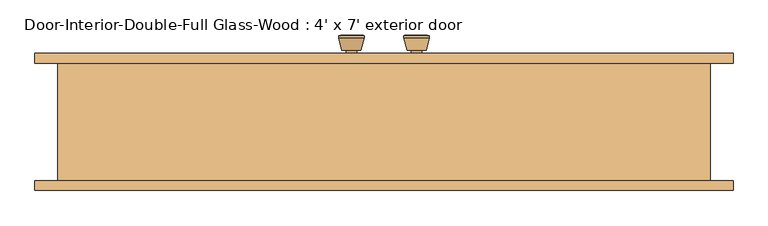
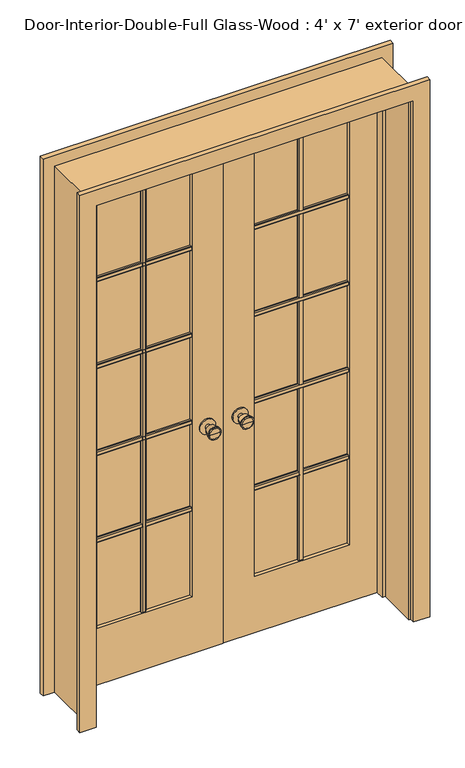
"""IFC4 building model written with IfcOpenShell, lengths in millimetres: door geometry, Door-Interior-Double-Full Glass-Wood : 4' x 7' exterior door."""

from ifc_helpers import new_model, si_unit, point, frame, frame_2d, origin, place, context, project, spatial, polyline, circle_curve, trimmed, segment, composite_curve, outline, extrude, faceted_brep, source, transform, mapped, element, save
from ifc_brep_helpers import plane_surface, cylinder_surface, revolved_surface, advanced_brep


def door_interior_double_full_glass_wood_4_x_7_exterior_door_6b6f14de(model_context):
    return source(origin(), model_context, "Body", "SolidModel", [
        advanced_brep(
        [(-63.5, 117.125, 914.4), (-73.5, 117.125, 914.4), (-53.5, 117.125, 914.4), (-83.9758676, 166.125, 914.4), (-63.5, 166.125, 914.4), (-43.0241324, 166.125, 914.4), (-88.5, 164.2971319, 914.4), (-38.5, 164.2971319, 914.4), (-88.5, 160.8334537, 914.4), (-38.5, 160.8334537, 914.4), (-82.136236, 136.125, 914.4), (-44.863764, 136.125, 914.4), (-73.5, 136.125, 914.4), (-53.5, 136.125, 914.4)],
        [
            (0, 1),
            (1, 2, circle_curve(frame((-63.5, 117.125, 914.4), z_axis=(0.0, -1.0, 0.0), x_axis=(1.0, 0.0, 0.0)), 10.0)),
            (2, 0),
            (2, 1, circle_curve(frame((-63.5, 117.125, 914.4), z_axis=(0.0, -1.0, 0.0), x_axis=(1.0, 0.0, 0.0)), 10.0)),
            (3, 4),
            (4, 5),
            (5, 3, circle_curve(frame((-63.5, 166.125, 914.4), z_axis=(0.0, 1.0, 0.0), x_axis=(1.0, 0.0, 0.0)), 20.4758676)),
            (3, 5, circle_curve(frame((-63.5, 166.125, 914.4), z_axis=(0.0, 1.0, 0.0), x_axis=(1.0, 0.0, 0.0)), 20.4758676)),
            (6, 3),
            (5, 7),
            (7, 6, circle_curve(frame((-63.5, 164.2971319, 914.4), z_axis=(0.0, 1.0, 0.0), x_axis=(1.0, 0.0, 0.0)), 25.0)),
            (6, 7, circle_curve(frame((-63.5, 164.2971319, 914.4), z_axis=(0.0, 1.0, 0.0), x_axis=(1.0, 0.0, 0.0)), 25.0)),
            (8, 6),
            (7, 9),
            (9, 8, circle_curve(frame((-63.5, 160.8334537, 914.4), z_axis=(0.0, 1.0, 0.0), x_axis=(1.0, 0.0, 0.0)), 25.0)),
            (8, 9, circle_curve(frame((-63.5, 160.8334537, 914.4), z_axis=(0.0, 1.0, 0.0), x_axis=(1.0, 0.0, 0.0)), 25.0)),
            (10, 8),
            (9, 11),
            (11, 10, circle_curve(frame((-63.5, 136.125, 914.4), z_axis=(0.0, 1.0, 0.0), x_axis=(1.0, 0.0, 0.0)), 18.636236)),
            (10, 11, circle_curve(frame((-63.5, 136.125, 914.4), z_axis=(0.0, 1.0, 0.0), x_axis=(1.0, 0.0, 0.0)), 18.636236)),
            (12, 10),
            (11, 13),
            (13, 12, circle_curve(frame((-63.5, 136.125, 914.4), z_axis=(0.0, 1.0, 0.0), x_axis=(1.0, 0.0, 0.0)), 10.0)),
            (12, 13, circle_curve(frame((-63.5, 136.125, 914.4), z_axis=(0.0, 1.0, 0.0), x_axis=(1.0, 0.0, 0.0)), 10.0)),
            (1, 12),
            (13, 2),
        ],
        [
            plane_surface(frame((-63.5, 117.125, 914.4), z_axis=(0.0, -1.0, 0.0), x_axis=(1.0, 0.0, 0.0))),
            plane_surface(frame((-63.5, 166.125, 914.4), z_axis=(0.0, 1.0, 0.0), x_axis=(1.0, 0.0, 0.0))),
            revolved_surface(polyline([(-43.0241324, 166.125, 914.4), (-38.5, 164.2971319, 914.4)]), (-63.5, 117.125, 914.4), (0.0, -1.0, 0.0)),
            cylinder_surface(frame((-63.5, 117.125, 914.4), z_axis=(0.0, -1.0, 0.0), x_axis=(1.0, 0.0, 0.0)), 25.0),
            revolved_surface(polyline([(-38.5, 160.8334537, 914.4), (-44.863764, 136.125, 914.4)]), (-63.5, 117.125, 914.4), (0.0, -1.0, 0.0)),
            plane_surface(frame((-63.5, 136.125, 914.4), z_axis=(0.0, -1.0, 0.0), x_axis=(1.0, 0.0, 0.0))),
            cylinder_surface(frame((-63.5, 117.125, 914.4), z_axis=(0.0, -1.0, 0.0), x_axis=(1.0, 0.0, 0.0)), 10.0),
        ],
        [
            (0, [[1, 2, 3]]),
            (0, [[-3, 4, -1]]),
            (1, [[5, 6, 7]]),
            (1, [[-6, -5, 8]]),
            (2, [[9, -7, 10, 11]]),
            (2, [[-10, -8, -9, 12]]),
            (3, [[13, -11, 14, 15]]),
            (3, [[-14, -12, -13, 16]]),
            (4, [[17, -15, 18, 19]]),
            (4, [[-18, -16, -17, 20]]),
            (5, [[21, -19, 22, 23]]),
            (5, [[-22, -20, -21, 24]]),
            (6, [[25, -23, 26, -2]]),
            (6, [[-26, -24, -25, -4]]),
        ],
    ),
        extrude(outline(composite_curve([segment(trimmed(circle_curve(frame_2d((914.4, -63.5)), 30.0), [point((914.4, -33.5))], [point((914.4, -93.5))], False, "CARTESIAN"), True, "CONTINUOUS"), segment(trimmed(circle_curve(frame_2d((914.4, -63.5)), 30.0), [point((914.4, -93.5))], [point((914.4, -33.5))], False, "CARTESIAN"), True, "CONTINUOUS")], self_intersect=False)), frame((0.0, 111.125, 0.0), z_axis=(0.0, 1.0, 0.0), x_axis=(0.0, 0.0, 1.0)), (0.0, 0.0, 1.0), 6.0),
        advanced_brep(
        [(-63.5, 70.2, 914.4), (-53.5, 70.2, 914.4), (-73.5, 70.2, 914.4), (-83.9758676, 21.2, 914.4), (-43.0241324, 21.2, 914.4), (-63.5, 21.2, 914.4), (-88.5, 23.0278681, 914.4), (-38.5, 23.0278681, 914.4), (-88.5, 26.4915463, 914.4), (-38.5, 26.4915463, 914.4), (-82.136236, 51.2, 914.4), (-44.863764, 51.2, 914.4), (-73.5, 51.2, 914.4), (-53.5, 51.2, 914.4)],
        [
            (0, 1),
            (1, 2, circle_curve(frame((-63.5, 70.2, 914.4), z_axis=(0.0, 1.0, 0.0), x_axis=(1.0, 0.0, 0.0)), 10.0)),
            (2, 0),
            (2, 1, circle_curve(frame((-63.5, 70.2, 914.4), z_axis=(0.0, 1.0, 0.0), x_axis=(1.0, 0.0, 0.0)), 10.0)),
            (3, 4, circle_curve(frame((-63.5, 21.2, 914.4), z_axis=(0.0, -1.0, 0.0), x_axis=(1.0, 0.0, 0.0)), 20.4758676)),
            (4, 5),
            (5, 3),
            (4, 3, circle_curve(frame((-63.5, 21.2, 914.4), z_axis=(0.0, -1.0, 0.0), x_axis=(1.0, 0.0, 0.0)), 20.4758676)),
            (6, 7, circle_curve(frame((-63.5, 23.0278681, 914.4), z_axis=(0.0, -1.0, 0.0), x_axis=(1.0, 0.0, 0.0)), 25.0)),
            (7, 4),
            (3, 6),
            (7, 6, circle_curve(frame((-63.5, 23.0278681, 914.4), z_axis=(0.0, -1.0, 0.0), x_axis=(1.0, 0.0, 0.0)), 25.0)),
            (8, 9, circle_curve(frame((-63.5, 26.4915463, 914.4), z_axis=(0.0, -1.0, 0.0), x_axis=(1.0, 0.0, 0.0)), 25.0)),
            (9, 7),
            (6, 8),
            (9, 8, circle_curve(frame((-63.5, 26.4915463, 914.4), z_axis=(0.0, -1.0, 0.0), x_axis=(1.0, 0.0, 0.0)), 25.0)),
            (10, 11, circle_curve(frame((-63.5, 51.2, 914.4), z_axis=(0.0, -1.0, 0.0), x_axis=(1.0, 0.0, 0.0)), 18.636236)),
            (11, 9),
            (8, 10),
            (11, 10, circle_curve(frame((-63.5, 51.2, 914.4), z_axis=(0.0, -1.0, 0.0), x_axis=(1.0, 0.0, 0.0)), 18.636236)),
            (12, 13, circle_curve(frame((-63.5, 51.2, 914.4), z_axis=(0.0, -1.0, 0.0), x_axis=(1.0, 0.0, 0.0)), 10.0)),
            (13, 11),
            (10, 12),
            (13, 12, circle_curve(frame((-63.5, 51.2, 914.4), z_axis=(0.0, -1.0, 0.0), x_axis=(1.0, 0.0, 0.0)), 10.0)),
            (1, 13),
            (12, 2),
        ],
        [
            plane_surface(frame((-63.5, 70.2, 914.4), z_axis=(0.0, 1.0, 0.0), x_axis=(1.0, 0.0, 0.0))),
            plane_surface(frame((-63.5, 21.2, 914.4), z_axis=(0.0, -1.0, 0.0), x_axis=(1.0, 0.0, 0.0))),
            revolved_surface(polyline([(-43.0241324, 21.2, 914.4), (-38.5, 23.0278681, 914.4)]), (-63.5, 70.2, 914.4), (0.0, 1.0, 0.0)),
            cylinder_surface(frame((-63.5, 70.2, 914.4), z_axis=(0.0, 1.0, 0.0), x_axis=(1.0, 0.0, 0.0)), 25.0),
            revolved_surface(polyline([(-38.5, 26.4915463, 914.4), (-44.863764, 51.2, 914.4)]), (-63.5, 70.2, 914.4), (0.0, 1.0, 0.0)),
            plane_surface(frame((-63.5, 51.2, 914.4), z_axis=(0.0, 1.0, 0.0), x_axis=(1.0, 0.0, 0.0))),
            cylinder_surface(frame((-63.5, 70.2, 914.4), z_axis=(0.0, 1.0, 0.0), x_axis=(1.0, 0.0, 0.0)), 10.0),
        ],
        [
            (0, [[1, 2, 3]]),
            (0, [[-3, 4, -1]]),
            (1, [[5, 6, 7]]),
            (1, [[8, -7, -6]]),
            (2, [[9, 10, -5, 11]]),
            (2, [[12, -11, -8, -10]]),
            (3, [[13, 14, -9, 15]]),
            (3, [[16, -15, -12, -14]]),
            (4, [[17, 18, -13, 19]]),
            (4, [[20, -19, -16, -18]]),
            (5, [[21, 22, -17, 23]]),
            (5, [[24, -23, -20, -22]]),
            (6, [[-2, 25, -21, 26]]),
            (6, [[-4, -26, -24, -25]]),
        ],
    ),
        extrude(outline(composite_curve([segment(trimmed(circle_curve(frame_2d((914.4, -63.5)), 30.0), [point((914.4, -33.5))], [point((914.4, -93.5))], False, "CARTESIAN"), True, "CONTINUOUS"), segment(trimmed(circle_curve(frame_2d((914.4, -63.5)), 30.0), [point((914.4, -93.5))], [point((914.4, -33.5))], False, "CARTESIAN"), True, "CONTINUOUS")], self_intersect=False)), frame((0.0, 70.2, 0.0), z_axis=(0.0, 1.0, 0.0), x_axis=(0.0, 0.0, 1.0)), (0.0, 0.0, 1.0), 6.0),
        extrude(outline(polyline([(90.17, 1667.51), (90.17, 1648.46), (83.82, 1648.46), (80.645, 1651.635), (80.645, 1664.335), (83.82, 1667.51), (90.17, 1667.51)])), frame((120.65, 0.0, 0.0), z_axis=(1.0, 0.0, 0.0), x_axis=(0.0, 1.0, 0.0)), (0.0, 0.0, 1.0), 368.3),
        extrude(outline(polyline([(90.17, 1310.9575), (90.17, 1291.9075), (83.82, 1291.9075), (80.645, 1295.0825), (80.645, 1307.7825), (83.82, 1310.9575), (90.17, 1310.9575)])), frame((120.65, 0.0, 0.0), z_axis=(1.0, 0.0, 0.0), x_axis=(0.0, 1.0, 0.0)), (0.0, 0.0, 1.0), 368.3),
        extrude(outline(polyline([(90.17, 954.405), (90.17, 935.355), (83.82, 935.355), (80.645, 938.53), (80.645, 951.23), (83.82, 954.405), (90.17, 954.405)])), frame((120.65, 0.0, 0.0), z_axis=(1.0, 0.0, 0.0), x_axis=(0.0, 1.0, 0.0)), (0.0, 0.0, 1.0), 368.3),
        extrude(outline(polyline([(295.275, 90.17), (314.325, 90.17), (314.325, 83.82), (311.15, 80.645), (298.45, 80.645), (295.275, 83.82), (295.275, 90.17)])), frame((0.0, 0.0, 231.775), z_axis=(0.0, 0.0, 1.0), x_axis=(1.0, 0.0, 0.0)), (0.0, 0.0, 1.0), 1782.7625),
        extrude(outline(polyline([(90.17, 597.8525), (90.17, 578.8025), (83.82, 578.8025), (80.645, 581.9775), (80.645, 594.6775), (83.82, 597.8525), (90.17, 597.8525)])), frame((120.65, 0.0, 0.0), z_axis=(1.0, 0.0, 0.0), x_axis=(0.0, 1.0, 0.0)), (0.0, 0.0, 1.0), 368.3),
        extrude(outline(polyline([(97.155, 1667.51), (103.505, 1667.51), (106.68, 1664.335), (106.68, 1651.635), (103.505, 1648.46), (97.155, 1648.46), (97.155, 1667.51)])), frame((-488.95, 0.0, 0.0), z_axis=(1.0, 0.0, 0.0), x_axis=(0.0, 1.0, 0.0)), (0.0, 0.0, 1.0), 368.3),
        extrude(outline(polyline([(97.155, 1310.9575), (103.505, 1310.9575), (106.68, 1307.7825), (106.68, 1295.0825), (103.505, 1291.9075), (97.155, 1291.9075), (97.155, 1310.9575)])), frame((-488.95, 0.0, 0.0), z_axis=(1.0, 0.0, 0.0), x_axis=(0.0, 1.0, 0.0)), (0.0, 0.0, 1.0), 368.3),
        extrude(outline(polyline([(97.155, 954.405), (103.505, 954.405), (106.68, 951.23), (106.68, 938.53), (103.505, 935.355), (97.155, 935.355), (97.155, 954.405)])), frame((-488.95, 0.0, 0.0), z_axis=(1.0, 0.0, 0.0), x_axis=(0.0, 1.0, 0.0)), (0.0, 0.0, 1.0), 368.3),
        extrude(outline(polyline([(-314.325, 97.155), (-314.325, 103.505), (-311.15, 106.68), (-298.45, 106.68), (-295.275, 103.505), (-295.275, 97.155), (-314.325, 97.155)])), frame((0.0, 0.0, 231.775), z_axis=(0.0, 0.0, 1.0), x_axis=(1.0, 0.0, 0.0)), (0.0, 0.0, 1.0), 1782.7625),
        extrude(outline(polyline([(97.155, 597.8525), (103.505, 597.8525), (106.68, 594.6775), (106.68, 581.9775), (103.505, 578.8025), (97.155, 578.8025), (97.155, 597.8525)])), frame((-488.95, 0.0, 0.0), z_axis=(1.0, 0.0, 0.0), x_axis=(0.0, 1.0, 0.0)), (0.0, 0.0, 1.0), 368.3),
        extrude(outline(polyline([(97.155, 1667.51), (103.505, 1667.51), (106.68, 1664.335), (106.68, 1651.635), (103.505, 1648.46), (97.155, 1648.46), (97.155, 1667.51)])), frame((120.65, 0.0, 0.0), z_axis=(1.0, 0.0, 0.0), x_axis=(0.0, 1.0, 0.0)), (0.0, 0.0, 1.0), 368.3),
        extrude(outline(polyline([(97.155, 1310.9575), (103.505, 1310.9575), (106.68, 1307.7825), (106.68, 1295.0825), (103.505, 1291.9075), (97.155, 1291.9075), (97.155, 1310.9575)])), frame((120.65, 0.0, 0.0), z_axis=(1.0, 0.0, 0.0), x_axis=(0.0, 1.0, 0.0)), (0.0, 0.0, 1.0), 368.3),
        extrude(outline(polyline([(97.155, 954.405), (103.505, 954.405), (106.68, 951.23), (106.68, 938.53), (103.505, 935.355), (97.155, 935.355), (97.155, 954.405)])), frame((120.65, 0.0, 0.0), z_axis=(1.0, 0.0, 0.0), x_axis=(0.0, 1.0, 0.0)), (0.0, 0.0, 1.0), 368.3),
        extrude(outline(polyline([(295.275, 97.155), (295.275, 103.505), (298.45, 106.68), (311.15, 106.68), (314.325, 103.505), (314.325, 97.155), (295.275, 97.155)])), frame((0.0, 0.0, 231.775), z_axis=(0.0, 0.0, 1.0), x_axis=(1.0, 0.0, 0.0)), (0.0, 0.0, 1.0), 1782.7625),
        extrude(outline(polyline([(97.155, 597.8525), (103.505, 597.8525), (106.68, 594.6775), (106.68, 581.9775), (103.505, 578.8025), (97.155, 578.8025), (97.155, 597.8525)])), frame((120.65, 0.0, 0.0), z_axis=(1.0, 0.0, 0.0), x_axis=(0.0, 1.0, 0.0)), (0.0, 0.0, 1.0), 368.3),
        extrude(outline(polyline([(90.17, 1667.51), (90.17, 1648.46), (83.82, 1648.46), (80.645, 1651.635), (80.645, 1664.335), (83.82, 1667.51), (90.17, 1667.51)])), frame((-488.95, 0.0, 0.0), z_axis=(1.0, 0.0, 0.0), x_axis=(0.0, 1.0, 0.0)), (0.0, 0.0, 1.0), 368.3),
        extrude(outline(polyline([(90.17, 1310.9575), (90.17, 1291.9075), (83.82, 1291.9075), (80.645, 1295.0825), (80.645, 1307.7825), (83.82, 1310.9575), (90.17, 1310.9575)])), frame((-488.95, 0.0, 0.0), z_axis=(1.0, 0.0, 0.0), x_axis=(0.0, 1.0, 0.0)), (0.0, 0.0, 1.0), 368.3),
        extrude(outline(polyline([(90.17, 954.405), (90.17, 935.355), (83.82, 935.355), (80.645, 938.53), (80.645, 951.23), (83.82, 954.405), (90.17, 954.405)])), frame((-488.95, 0.0, 0.0), z_axis=(1.0, 0.0, 0.0), x_axis=(0.0, 1.0, 0.0)), (0.0, 0.0, 1.0), 368.3),
        extrude(outline(polyline([(-314.325, 90.17), (-295.275, 90.17), (-295.275, 83.82), (-298.45, 80.645), (-311.15, 80.645), (-314.325, 83.82), (-314.325, 90.17)])), frame((0.0, 0.0, 231.775), z_axis=(0.0, 0.0, 1.0), x_axis=(1.0, 0.0, 0.0)), (0.0, 0.0, 1.0), 1782.7625),
        extrude(outline(polyline([(90.17, 597.8525), (90.17, 578.8025), (83.82, 578.8025), (80.645, 581.9775), (80.645, 594.6775), (83.82, 597.8525), (90.17, 597.8525)])), frame((-488.95, 0.0, 0.0), z_axis=(1.0, 0.0, 0.0), x_axis=(0.0, 1.0, 0.0)), (0.0, 0.0, 1.0), 368.3),
        advanced_brep(
        [(63.5, 70.2, 914.4), (73.5, 70.2, 914.4), (53.5, 70.2, 914.4), (83.9758676, 21.2, 914.4), (63.5, 21.2, 914.4), (43.0241324, 21.2, 914.4), (88.5, 23.0278681, 914.4), (38.5, 23.0278681, 914.4), (88.5, 26.4915463, 914.4), (38.5, 26.4915463, 914.4), (82.136236, 51.2, 914.4), (44.863764, 51.2, 914.4), (73.5, 51.2, 914.4), (53.5, 51.2, 914.4)],
        [
            (0, 1),
            (1, 2, circle_curve(frame((63.5, 70.2, 914.4), z_axis=(0.0, 1.0, 0.0), x_axis=(-1.0, 0.0, 0.0)), 10.0)),
            (2, 0),
            (2, 1, circle_curve(frame((63.5, 70.2, 914.4), z_axis=(0.0, 1.0, 0.0), x_axis=(-1.0, 0.0, 0.0)), 10.0)),
            (3, 4),
            (4, 5),
            (5, 3, circle_curve(frame((63.5, 21.2, 914.4), z_axis=(0.0, -1.0, 0.0), x_axis=(-1.0, 0.0, 0.0)), 20.4758676)),
            (3, 5, circle_curve(frame((63.5, 21.2, 914.4), z_axis=(0.0, -1.0, 0.0), x_axis=(-1.0, 0.0, 0.0)), 20.4758676)),
            (6, 3),
            (5, 7),
            (7, 6, circle_curve(frame((63.5, 23.0278681, 914.4), z_axis=(0.0, -1.0, 0.0), x_axis=(-1.0, 0.0, 0.0)), 25.0)),
            (6, 7, circle_curve(frame((63.5, 23.0278681, 914.4), z_axis=(0.0, -1.0, 0.0), x_axis=(-1.0, 0.0, 0.0)), 25.0)),
            (8, 6),
            (7, 9),
            (9, 8, circle_curve(frame((63.5, 26.4915463, 914.4), z_axis=(0.0, -1.0, 0.0), x_axis=(-1.0, 0.0, 0.0)), 25.0)),
            (8, 9, circle_curve(frame((63.5, 26.4915463, 914.4), z_axis=(0.0, -1.0, 0.0), x_axis=(-1.0, 0.0, 0.0)), 25.0)),
            (10, 8),
            (9, 11),
            (11, 10, circle_curve(frame((63.5, 51.2, 914.4), z_axis=(0.0, -1.0, 0.0), x_axis=(-1.0, 0.0, 0.0)), 18.636236)),
            (10, 11, circle_curve(frame((63.5, 51.2, 914.4), z_axis=(0.0, -1.0, 0.0), x_axis=(-1.0, 0.0, 0.0)), 18.636236)),
            (12, 10),
            (11, 13),
            (13, 12, circle_curve(frame((63.5, 51.2, 914.4), z_axis=(0.0, -1.0, 0.0), x_axis=(-1.0, 0.0, 0.0)), 10.0)),
            (12, 13, circle_curve(frame((63.5, 51.2, 914.4), z_axis=(0.0, -1.0, 0.0), x_axis=(-1.0, 0.0, 0.0)), 10.0)),
            (1, 12),
            (13, 2),
        ],
        [
            plane_surface(frame((63.5, 70.2, 914.4), z_axis=(0.0, 1.0, 0.0), x_axis=(-1.0, 0.0, 0.0))),
            plane_surface(frame((63.5, 21.2, 914.4), z_axis=(0.0, -1.0, 0.0), x_axis=(-1.0, 0.0, 0.0))),
            revolved_surface(polyline([(43.0241324, 21.2, 914.4), (38.5, 23.0278681, 914.4)]), (63.5, 70.2, 914.4), (0.0, 1.0, 0.0)),
            cylinder_surface(frame((63.5, 70.2, 914.4), z_axis=(0.0, 1.0, 0.0), x_axis=(-1.0, 0.0, 0.0)), 25.0),
            revolved_surface(polyline([(38.5, 26.4915463, 914.4), (44.863764, 51.2, 914.4)]), (63.5, 70.2, 914.4), (0.0, 1.0, 0.0)),
            plane_surface(frame((63.5, 51.2, 914.4), z_axis=(0.0, 1.0, 0.0), x_axis=(-1.0, 0.0, 0.0))),
            cylinder_surface(frame((63.5, 70.2, 914.4), z_axis=(0.0, 1.0, 0.0), x_axis=(-1.0, 0.0, 0.0)), 10.0),
        ],
        [
            (0, [[1, 2, 3]]),
            (0, [[-3, 4, -1]]),
            (1, [[5, 6, 7]]),
            (1, [[-6, -5, 8]]),
            (2, [[9, -7, 10, 11]]),
            (2, [[-10, -8, -9, 12]]),
            (3, [[13, -11, 14, 15]]),
            (3, [[-14, -12, -13, 16]]),
            (4, [[17, -15, 18, 19]]),
            (4, [[-18, -16, -17, 20]]),
            (5, [[21, -19, 22, 23]]),
            (5, [[-22, -20, -21, 24]]),
            (6, [[25, -23, 26, -2]]),
            (6, [[-26, -24, -25, -4]]),
        ],
    ),
        extrude(outline(composite_curve([segment(trimmed(circle_curve(frame_2d((914.4, 63.5)), 30.0), [point((914.4, 33.5))], [point((914.4, 93.5))], False, "CARTESIAN"), True, "CONTINUOUS"), segment(trimmed(circle_curve(frame_2d((914.4, 63.5)), 30.0), [point((914.4, 93.5))], [point((914.4, 33.5))], False, "CARTESIAN"), True, "CONTINUOUS")], self_intersect=False)), frame((0.0, 70.2, 0.0), z_axis=(0.0, 1.0, 0.0), x_axis=(0.0, 0.0, 1.0)), (0.0, 0.0, 1.0), 6.0),
        advanced_brep(
        [(63.5, 117.125, 914.4), (53.5, 117.125, 914.4), (73.5, 117.125, 914.4), (83.9758676, 166.125, 914.4), (43.0241324, 166.125, 914.4), (63.5, 166.125, 914.4), (88.5, 164.2971319, 914.4), (38.5, 164.2971319, 914.4), (88.5, 160.8334537, 914.4), (38.5, 160.8334537, 914.4), (82.136236, 136.125, 914.4), (44.863764, 136.125, 914.4), (73.5, 136.125, 914.4), (53.5, 136.125, 914.4)],
        [
            (0, 1),
            (1, 2, circle_curve(frame((63.5, 117.125, 914.4), z_axis=(0.0, -1.0, 0.0), x_axis=(-1.0, 0.0, 0.0)), 10.0)),
            (2, 0),
            (2, 1, circle_curve(frame((63.5, 117.125, 914.4), z_axis=(0.0, -1.0, 0.0), x_axis=(-1.0, 0.0, 0.0)), 10.0)),
            (3, 4, circle_curve(frame((63.5, 166.125, 914.4), z_axis=(0.0, 1.0, 0.0), x_axis=(-1.0, 0.0, 0.0)), 20.4758676)),
            (4, 5),
            (5, 3),
            (4, 3, circle_curve(frame((63.5, 166.125, 914.4), z_axis=(0.0, 1.0, 0.0), x_axis=(-1.0, 0.0, 0.0)), 20.4758676)),
            (6, 7, circle_curve(frame((63.5, 164.2971319, 914.4), z_axis=(0.0, 1.0, 0.0), x_axis=(-1.0, 0.0, 0.0)), 25.0)),
            (7, 4),
            (3, 6),
            (7, 6, circle_curve(frame((63.5, 164.2971319, 914.4), z_axis=(0.0, 1.0, 0.0), x_axis=(-1.0, 0.0, 0.0)), 25.0)),
            (8, 9, circle_curve(frame((63.5, 160.8334537, 914.4), z_axis=(0.0, 1.0, 0.0), x_axis=(-1.0, 0.0, 0.0)), 25.0)),
            (9, 7),
            (6, 8),
            (9, 8, circle_curve(frame((63.5, 160.8334537, 914.4), z_axis=(0.0, 1.0, 0.0), x_axis=(-1.0, 0.0, 0.0)), 25.0)),
            (10, 11, circle_curve(frame((63.5, 136.125, 914.4), z_axis=(0.0, 1.0, 0.0), x_axis=(-1.0, 0.0, 0.0)), 18.636236)),
            (11, 9),
            (8, 10),
            (11, 10, circle_curve(frame((63.5, 136.125, 914.4), z_axis=(0.0, 1.0, 0.0), x_axis=(-1.0, 0.0, 0.0)), 18.636236)),
            (12, 13, circle_curve(frame((63.5, 136.125, 914.4), z_axis=(0.0, 1.0, 0.0), x_axis=(-1.0, 0.0, 0.0)), 10.0)),
            (13, 11),
            (10, 12),
            (13, 12, circle_curve(frame((63.5, 136.125, 914.4), z_axis=(0.0, 1.0, 0.0), x_axis=(-1.0, 0.0, 0.0)), 10.0)),
            (1, 13),
            (12, 2),
        ],
        [
            plane_surface(frame((63.5, 117.125, 914.4), z_axis=(0.0, -1.0, 0.0), x_axis=(-1.0, 0.0, 0.0))),
            plane_surface(frame((63.5, 166.125, 914.4), z_axis=(0.0, 1.0, 0.0), x_axis=(-1.0, 0.0, 0.0))),
            revolved_surface(polyline([(43.0241324, 166.125, 914.4), (38.5, 164.2971319, 914.4)]), (63.5, 117.125, 914.4), (0.0, -1.0, 0.0)),
            cylinder_surface(frame((63.5, 117.125, 914.4), z_axis=(0.0, -1.0, 0.0), x_axis=(-1.0, 0.0, 0.0)), 25.0),
            revolved_surface(polyline([(38.5, 160.8334537, 914.4), (44.863764, 136.125, 914.4)]), (63.5, 117.125, 914.4), (0.0, -1.0, 0.0)),
            plane_surface(frame((63.5, 136.125, 914.4), z_axis=(0.0, -1.0, 0.0), x_axis=(-1.0, 0.0, 0.0))),
            cylinder_surface(frame((63.5, 117.125, 914.4), z_axis=(0.0, -1.0, 0.0), x_axis=(-1.0, 0.0, 0.0)), 10.0),
        ],
        [
            (0, [[1, 2, 3]]),
            (0, [[-3, 4, -1]]),
            (1, [[5, 6, 7]]),
            (1, [[8, -7, -6]]),
            (2, [[9, 10, -5, 11]]),
            (2, [[12, -11, -8, -10]]),
            (3, [[13, 14, -9, 15]]),
            (3, [[16, -15, -12, -14]]),
            (4, [[17, 18, -13, 19]]),
            (4, [[20, -19, -16, -18]]),
            (5, [[21, 22, -17, 23]]),
            (5, [[24, -23, -20, -22]]),
            (6, [[-2, 25, -21, 26]]),
            (6, [[-4, -26, -24, -25]]),
        ],
    ),
        extrude(outline(composite_curve([segment(trimmed(circle_curve(frame_2d((914.4, 63.5)), 30.0), [point((914.4, 33.5))], [point((914.4, 93.5))], False, "CARTESIAN"), True, "CONTINUOUS"), segment(trimmed(circle_curve(frame_2d((914.4, 63.5)), 30.0), [point((914.4, 93.5))], [point((914.4, 33.5))], False, "CARTESIAN"), True, "CONTINUOUS")], self_intersect=False)), frame((0.0, 111.125, 0.0), z_axis=(0.0, 1.0, 0.0), x_axis=(0.0, 0.0, 1.0)), (0.0, 0.0, 1.0), 6.0),
        extrude(outline(polyline([(0.0, 615.95), (0.0, 679.45), (2203.45, 679.45), (2203.45, -679.45), (0.0, -679.45), (0.0, -615.95), (2139.95, -615.95), (2139.95, 615.95), (0.0, 615.95)])), frame((0.0, -136.525, 0.0), z_axis=(0.0, 1.0, 0.0), x_axis=(0.0, 0.0, 1.0)), (0.0, 0.0, 1.0), 19.05),
        extrude(outline(polyline([(0.0, 615.95), (0.0, 679.45), (2203.45, 679.45), (2203.45, -679.45), (0.0, -679.45), (0.0, -615.95), (2139.95, -615.95), (2139.95, 615.95), (0.0, 615.95)])), frame((0.0, 111.125, 0.0), z_axis=(0.0, 1.0, 0.0), x_axis=(0.0, 0.0, 1.0)), (0.0, 0.0, 1.0), 19.05),
        faceted_brep([(635.0, 111.125, 0.0), (635.0, -117.475, 0.0), (609.6, -117.475, 0.0), (609.6, 41.275, 0.0), (596.9, 41.275, 0.0), (596.9, 76.2, 0.0), (609.6, 76.2, 0.0), (609.6, 111.125, 0.0), (635.0, 111.125, 2159.0), (635.0, -117.475, 2159.0), (-635.0, -117.475, 2159.0), (-635.0, -117.475, 0.0), (-609.6, -117.475, 0.0), (-609.6, -117.475, 2133.6), (609.6, -117.475, 2133.6), (609.6, 41.275, 2133.6), (-609.6, 41.275, 2133.6), (-609.6, 41.275, 0.0), (-596.9, 41.275, 0.0), (-596.9, 41.275, 2120.9), (596.9, 41.275, 2120.9), (596.9, 76.2, 2120.9), (1.5875, 76.2, 2120.9), (-1.6019111, 76.2, 2120.9), (-596.9, 76.2, 2120.9), (-596.9, 76.2, 0.0), (-609.6, 76.2, 0.0), (-609.6, 76.2, 2133.6), (-1.6019111, 76.2, 2133.6), (1.5875, 76.2, 2133.6), (609.6, 76.2, 2133.6), (609.6, 111.125, 2133.6), (1.5875, 111.125, 2133.6), (-1.6019111, 111.125, 2133.6), (-609.6, 111.125, 2133.6), (-609.6, 111.125, 0.0), (-635.0, 111.125, 0.0), (-635.0, 111.125, 2159.0)], [[[0, 1, 2, 3, 4, 5, 6, 7]], [[1, 0, 8, 9]], [[2, 1, 9, 10, 11, 12, 13, 14]], [[3, 2, 14, 15]], [[4, 3, 15, 16, 17, 18, 19, 20]], [[5, 4, 20, 21]], [[6, 5, 21, 22, 23, 24, 25, 26, 27, 28, 29, 30]], [[7, 6, 30, 31]], [[0, 7, 31, 32, 33, 34, 35, 36, 37, 8]], [[9, 8, 37, 10]], [[14, 13, 16, 15]], [[20, 19, 24, 23, 22, 21]], [[31, 30, 29, 28, 27, 34, 33, 32]], [[12, 11, 36, 35, 26, 25, 18, 17]], [[11, 10, 37, 36]], [[13, 12, 17, 16]], [[19, 18, 25, 24]], [[27, 26, 35, 34]]]),
        extrude(outline(polyline([(2133.6, -609.6), (0.0, -609.6), (0.0, -1.6019111), (2133.6, -1.6019111), (2133.6, -609.6)]), holes=[polyline([(231.775, -488.95), (2014.5375, -488.95), (2014.5375, -120.65), (231.775, -120.65), (231.775, -488.95)])]), frame((0.0, 76.2, 0.0), z_axis=(0.0, 1.0, 0.0), x_axis=(0.0, 0.0, 1.0)), (0.0, 0.0, 1.0), 34.925),
        extrude(outline(polyline([(0.0, 609.6), (2133.6, 609.6), (2133.6, 1.5875), (0.0, 1.5875), (0.0, 609.6)]), holes=[polyline([(2014.5375, 120.65), (2014.5375, 488.95), (231.775, 488.95), (231.775, 120.65), (2014.5375, 120.65)])]), frame((0.0, 76.2, 0.0), z_axis=(0.0, 1.0, 0.0), x_axis=(0.0, 0.0, 1.0)), (0.0, 0.0, 1.0), 34.925),
        extrude(outline(polyline([(488.95, 90.17), (120.65, 90.17), (120.65, 97.155), (488.95, 97.155), (488.95, 90.17)])), frame((0.0, 0.0, 231.775), z_axis=(0.0, 0.0, 1.0), x_axis=(1.0, 0.0, 0.0)), (0.0, 0.0, 1.0), 1782.7625),
        extrude(outline(polyline([(-120.65, 90.17), (-488.95, 90.17), (-488.95, 97.155), (-120.65, 97.155), (-120.65, 90.17)])), frame((0.0, 0.0, 231.775), z_axis=(0.0, 0.0, 1.0), x_axis=(1.0, 0.0, 0.0)), (0.0, 0.0, 1.0), 1782.7625),
    ])


if __name__ == "__main__":
    model = new_model("IFC4")
    model_context = context("Model", 3, world=origin())
    ifc_project = project(units=[si_unit("LENGTHUNIT", "METRE", prefix="MILLI")], contexts=[model_context])
    site = spatial("IfcSite", under=ifc_project)
    building = spatial("IfcBuilding", under=site)
    placement = place(None, origin())
    door_interior_double_full_glass_wood_4_x_7_exterior_door_shape = door_interior_double_full_glass_wood_4_x_7_exterior_door_6b6f14de(model_context)
    element("IfcDoor", 1, ObjectType="Door-Interior-Double-Full Glass-Wood : 4' x 7' exterior door", at=placement, inside=building, context=model_context, shape_type="MappedRepresentation", body=[
        mapped(door_interior_double_full_glass_wood_4_x_7_exterior_door_shape, transform((0.0, 0.0, 0.0), x_axis=(1.0, 0.0, 0.0), y_axis=(0.0, 1.0, 0.0), z_axis=(0.0, 0.0, 1.0))),
    ])
    save(model, "model.ifc")

# Revit data of these elements
# Type "Door-Interior-Double-Full Glass-Wood : 4' x 7' exterior door"
#   Type Mark = "9"
#   Assembly Code = "C1020300"
#   Analytic Construction = "French door, wood frame with single glass"
#   Top Rail = 0' - 4 11/16"
#   Thickness = 0' - 1 3/8"
#   Thermal Resistance (R) = 1.0696 (h·ft²·°F)/BTU
#   Swing Angle [instance default] = 90.00°
#   Stiles = 0' - 4 3/4"
#   Rough Width = 4' - 2"
#   Rough Height = 7' - 1"
#   Panel Width = 2' - 0"
#   Height = 7' - 0"
#   Width = 4' - 0"
#   Heat Transfer Coefficient (U) = 0.9350 BTU/(h·ft²·°F)
#   Bottom Rail = 0' - 9 1/8"
#   Show Grill [instance default] = yes
#   Trim Material = Cherry
#   Panel Material = Cherry
#   Frame Material = Cherry
#   Door Handle Material = Aluminum
#   Visual Light Transmittance = 0
#   Solar Heat Gain Coefficient = 0
#   Wall Closure = (empty or 0)
#   Function = (empty or 0)
# Element 1 (IfcDoor, "Door-Interior-Double-Full Glass-Wood : 4' x 7' exterior door")
#   Materials on its faces: "Cherry", "Aluminum", "Glass"
# Materials
#   "Cherry": class "Wood", colour RGB 226 177 128, transparency 0, Description = "Prunus Serotina", Cost = 0
#   "Aluminum": class "Metal", colour RGB 247 247 247, transparency 0, Description = "Aluminum 6061", Cost = 0
#   "Glass": class "Glass", colour RGB 0 128 192, transparency 0.75, Description = "Soda Lime Glass", Cost = 0
